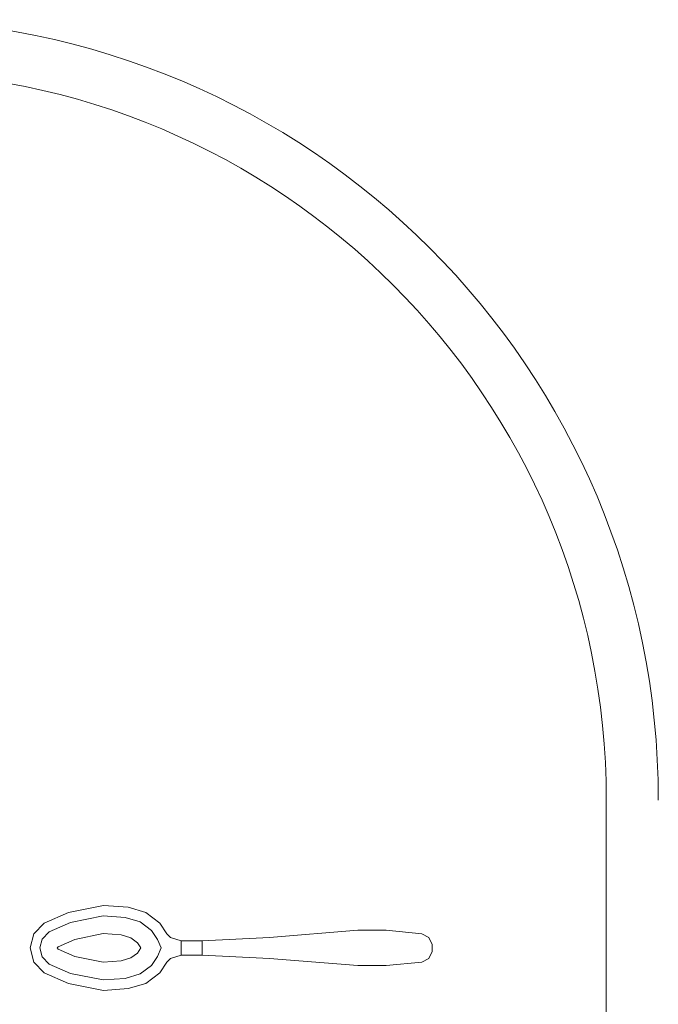
# Model space of a CAD drawing. Units: inches. Extents: x 375 to 1122, y 27 to 1069.
# Tile 147 of 155: x 737.5 to 747.02, y 901.85 to 916.52. Entities that reach past the tile are written whole.
import ezdxf

# ---------------------------------------------------------------- set-up
doc = ezdxf.new("R2010")
doc.units = ezdxf.units.IN
doc.layers.add('A-ANNO-DIMS', color=2, linetype='Continuous', lineweight=18)
doc.layers.add('Furniture', color=30, linetype='Continuous', lineweight=18)
doc.styles.get("Standard").update_dxf_attribs({"font": 'arial.ttf'})
doc.dimstyles.new('ISO-25', dxfattribs={"dimtxt": 12, "dimasz": 2.5, "dimexe": 1.5, "dimexo": 1.5, "dimtad": 1, "dimdec": 1, "dimlunit": 3, "dimtxsty": 'Standard', "dimblk": 'ARCHTICK', "dimcen": 2.5, "dimadec": 0, "dimazin": 0, "dimtfac": 1, "dimtdec": 1, "dimtmove": 0, "dimatfit": 3, "dimfxl": 1.5, "dimfxlon": 1, "dimarcsym": 0})

# ---------------------------------------------------------------- blocks, each defined once
blk = doc.blocks.new('A$C403C54AD')
blk.add_line((0.83575, 1.53256, -0.0006), (1.99923, 1.53256, -0.0006))
for radius in [0.29087, 0.27148]:
    blk.add_arc((0.83575, 1.26108, -0.0006), radius, 90, 180)
for points, invisible_edges in [([(0.88693, 1.46634, -0.04237), (0.89484, 1.46634, -0.04237), (0.89616, 1.4637, -0.04257), (0.88561, 1.4637, -0.04257)], 5), ([(0.88693, 1.46634, -0.04634), (0.89484, 1.46634, -0.04634), (0.89616, 1.4637, -0.04655), (0.88561, 1.4637, -0.04655)], 5), ([(0.8922, 1.46766, -0.04251), (0.88956, 1.46766, -0.04251), (0.88693, 1.46634, -0.04237), (0.89484, 1.46634, -0.04237)], 4), ([(0.8922, 1.46766, -0.04605), (0.88956, 1.46766, -0.04605), (0.88693, 1.46634, -0.04634), (0.89484, 1.46634, -0.04634)], 4), ([(0.89616, 1.4637, -0.04257), (0.88561, 1.4637, -0.04257), (0.88429, 1.45051, -0.0426), (0.89748, 1.45051, -0.0426)], 5), ([(0.89616, 1.4637, -0.04655), (0.88561, 1.4637, -0.04655), (0.88429, 1.45051, -0.04658), (0.89748, 1.45051, -0.04658)], 5), ([(0.88429, 1.45051, -0.0426), (0.89748, 1.45051, -0.0426), (0.89748, 1.43995, -0.04232), (0.88429, 1.43995, -0.04232)], 5), ([(0.88429, 1.45051, -0.04658), (0.89748, 1.45051, -0.04658), (0.89748, 1.43995, -0.0463), (0.88429, 1.43995, -0.0463)], 5), ([(0.89748, 1.43995, -0.0463), (0.88429, 1.43995, -0.0463), (0.88693, 1.40697, -0.04292), (0.89484, 1.40697, -0.04292)], 5), ([(0.88429, 1.43995, -0.0463), (0.88429, 1.43995, -0.04232), (0.88693, 1.40697, -0.04028), (0.88693, 1.40697, -0.04292)], 4), ([(0.89748, 1.43995, -0.04232), (0.88429, 1.43995, -0.04232), (0.88693, 1.40697, -0.04028), (0.89484, 1.40697, -0.04028)], 5), ([(0.89484, 1.40697, -0.04292), (0.89484, 1.40697, -0.04028), (0.89748, 1.43995, -0.04232), (0.89748, 1.43995, -0.0463)], 1), ([(0.88693, 1.40697, -0.04028), (0.89484, 1.40697, -0.04028), (0.89352, 1.3819, -0.03779), (0.88825, 1.3819, -0.03779)], 1), ([(0.88693, 1.40697, -0.04028), (0.88693, 1.40697, -0.04292), (0.88825, 1.3819, -0.04001), (0.88825, 1.3819, -0.03779)], 5), ([(0.88693, 1.40697, -0.04292), (0.89484, 1.40697, -0.04292), (0.89352, 1.3819, -0.04001), (0.88825, 1.3819, -0.04001)], 1), ([(0.89352, 1.3819, -0.03779), (0.89352, 1.3819, -0.04001), (0.89484, 1.40697, -0.04292), (0.89484, 1.40697, -0.04028)], 5), ([(0.88825, 1.3819, -0.04001), (0.88825, 1.3819, -0.03779), (0.88825, 1.37399, -0.03842), (0.88825, 1.37399, -0.04064)], 5), ([(0.89352, 1.37399, -0.04064), (0.89352, 1.37399, -0.03842), (0.89352, 1.3819, -0.03779), (0.89352, 1.3819, -0.04001)], 5), ([(0.88825, 1.37399, -0.03842), (0.89352, 1.37399, -0.03842), (0.89484, 1.37003, -0.04027), (0.88693, 1.37003, -0.04027)], 4), ([(0.88825, 1.37399, -0.03842), (0.88825, 1.37399, -0.04064), (0.88693, 1.37003, -0.04236), (0.88693, 1.37003, -0.04027)], 5), ([(0.88825, 1.37399, -0.04064), (0.89352, 1.37399, -0.04064), (0.89484, 1.37003, -0.04236), (0.88693, 1.37003, -0.04236)], 4), ([(0.89352, 1.37399, -0.04064), (0.89352, 1.37399, -0.03842), (0.89484, 1.37003, -0.04027), (0.89484, 1.37003, -0.04236)], 5), ([(0.89484, 1.37003, -0.04027), (0.88693, 1.37003, -0.04027), (0.88561, 1.3687, -0.041), (0.89616, 1.3687, -0.041)], 5), ([(0.89484, 1.37003, -0.04236), (0.88693, 1.37003, -0.04236), (0.88561, 1.3687, -0.04315), (0.89616, 1.3687, -0.04315)], 5), ([(0.88693, 1.37003, -0.04236), (0.88693, 1.37003, -0.04027), (0.88561, 1.3687, -0.041), (0.88561, 1.3687, -0.04315)], 1), ([(0.89484, 1.37003, -0.04027), (0.89484, 1.37003, -0.04236), (0.89616, 1.3687, -0.04315), (0.89616, 1.3687, -0.041)], 1), ([(0.88165, 1.36608, -0.04195), (0.88434, 1.36289, -0.04423), (0.88119, 1.35867, -0.04406), (0.87769, 1.36082, -0.04147)], 5), ([(0.88165, 1.36608, -0.04063), (0.88434, 1.36289, -0.04291), (0.88119, 1.35867, -0.04274), (0.87769, 1.36082, -0.04015)], 5), ([(0.88774, 1.36518, -0.04424), (0.88561, 1.3687, -0.04315), (0.88165, 1.36608, -0.04195), (0.88434, 1.36289, -0.04423)], 5), ([(0.88774, 1.36518, -0.04292), (0.88561, 1.3687, -0.041), (0.88165, 1.36608, -0.04063), (0.88434, 1.36289, -0.04291)], 5), ([(0.88561, 1.3687, -0.04315), (0.89088, 1.3687, -0.04315), (0.89088, 1.36654, -0.04406), (0.88774, 1.36518, -0.04424)], 11), ([(0.88561, 1.3687, -0.041), (0.89088, 1.3687, -0.041), (0.89088, 1.36654, -0.04274), (0.88774, 1.36518, -0.04292)], 11), ([(0.88774, 1.36518, -0.04424), (0.89088, 1.35902, -0.04627), (0.89088, 1.35902, -0.04627), (0.89088, 1.36654, -0.04406)], 5), ([(0.88774, 1.36518, -0.04292), (0.89088, 1.35902, -0.04495), (0.89088, 1.35902, -0.04495), (0.89088, 1.36654, -0.04274)], 5), ([(0.89616, 1.3687, -0.04315), (0.89088, 1.3687, -0.04315), (0.89088, 1.36654, -0.04406), (0.89402, 1.36518, -0.04424)], 11), ([(0.89616, 1.3687, -0.041), (0.89088, 1.3687, -0.041), (0.89088, 1.36654, -0.04274), (0.89402, 1.36518, -0.04292)], 11), ([(0.89402, 1.36518, -0.04424), (0.89088, 1.35902, -0.04627), (0.89088, 1.35902, -0.04627), (0.89088, 1.36654, -0.04406)], 5), ([(0.89402, 1.36518, -0.04292), (0.89088, 1.35902, -0.04495), (0.89088, 1.35902, -0.04495), (0.89088, 1.36654, -0.04274)], 5), ([(0.89402, 1.36518, -0.04292), (0.89616, 1.3687, -0.041), (0.90012, 1.36608, -0.04063), (0.89743, 1.36289, -0.04291)], 5), ([(0.90012, 1.36608, -0.04195), (0.89743, 1.36289, -0.04423), (0.90058, 1.35867, -0.04406), (0.90408, 1.36082, -0.04147)], 5), ([(0.90012, 1.36608, -0.04063), (0.89743, 1.36289, -0.04291), (0.90058, 1.35867, -0.04274), (0.90408, 1.36082, -0.04015)], 5), ([(0.88119, 1.35867, -0.04406), (0.88715, 1.3553, -0.04638), (0.88892, 1.35767, -0.04647), (0.88434, 1.36289, -0.04423)], 5), ([(0.88119, 1.35867, -0.04274), (0.88715, 1.3553, -0.04506), (0.88892, 1.35767, -0.04515), (0.88434, 1.36289, -0.04291)], 5), ([(0.88892, 1.35767, -0.04647), (0.88434, 1.36289, -0.04423), (0.88774, 1.36518, -0.04424), (0.89088, 1.35902, -0.04627)], 5), ([(0.88892, 1.35767, -0.04515), (0.88434, 1.36289, -0.04291), (0.88774, 1.36518, -0.04292), (0.89088, 1.35902, -0.04495)], 5), ([(0.89284, 1.35767, -0.04647), (0.89743, 1.36289, -0.04423), (0.89402, 1.36518, -0.04424), (0.89088, 1.35902, -0.04627)], 5), ([(0.89284, 1.35767, -0.04515), (0.89743, 1.36289, -0.04291), (0.89402, 1.36518, -0.04292), (0.89088, 1.35902, -0.04495)], 5), ([(0.90058, 1.35867, -0.04406), (0.89462, 1.3553, -0.04638), (0.89284, 1.35767, -0.04647), (0.89743, 1.36289, -0.04423)], 5), ([(0.90058, 1.35867, -0.04274), (0.89462, 1.3553, -0.04506), (0.89284, 1.35767, -0.04515), (0.89743, 1.36289, -0.04291)], 5), ([(0.88119, 1.35867, -0.04274), (0.87769, 1.36082, -0.04015), (0.87571, 1.35422, -0.03974), (0.87953, 1.35316, -0.04222)], 5), ([(0.88119, 1.35867, -0.04406), (0.87769, 1.36082, -0.04147), (0.87571, 1.35422, -0.04106), (0.87953, 1.35316, -0.04354)], 5), ([(0.88604, 1.35158, -0.04614), (0.87953, 1.35316, -0.04354), (0.88119, 1.35867, -0.04406), (0.88715, 1.3553, -0.04638)], 5), ([(0.88604, 1.35158, -0.04482), (0.87953, 1.35316, -0.04222), (0.88119, 1.35867, -0.04274), (0.88715, 1.3553, -0.04506)], 5), ([(0.88892, 1.35767, -0.04647), (0.89284, 1.35767, -0.04647), (0.89088, 1.35902, -0.04627)], 1), ([(0.88892, 1.35767, -0.04515), (0.89284, 1.35767, -0.04515), (0.89088, 1.35902, -0.04495)], 1), ([(0.89573, 1.35158, -0.04482), (0.90224, 1.35316, -0.04222), (0.90058, 1.35867, -0.04274), (0.89462, 1.3553, -0.04506)], 5), ([(0.90058, 1.35867, -0.04274), (0.90408, 1.36082, -0.04015), (0.90606, 1.35422, -0.03974), (0.90224, 1.35316, -0.04222)], 5), ([(0.90058, 1.35867, -0.04406), (0.90408, 1.36082, -0.04147), (0.90606, 1.35422, -0.04106), (0.90224, 1.35316, -0.04354)], 5), ([(0.88604, 1.35158, -0.04614), (0.89573, 1.35158, -0.04614), (0.89462, 1.3553, -0.04638), (0.88715, 1.3553, -0.04638)], 5), ([(0.88604, 1.35158, -0.04482), (0.89573, 1.35158, -0.04482), (0.89462, 1.3553, -0.04506), (0.88715, 1.3553, -0.04506)], 5), ([(0.89462, 1.3553, -0.04638), (0.88715, 1.3553, -0.04638), (0.88892, 1.35767, -0.04647), (0.89284, 1.35767, -0.04647)], 5), ([(0.89462, 1.3553, -0.04506), (0.88715, 1.3553, -0.04506), (0.88892, 1.35767, -0.04515), (0.89284, 1.35767, -0.04515)], 5), ([(0.87571, 1.35422, -0.03974), (0.87953, 1.35316, -0.04222), (0.87893, 1.34491, -0.04133), (0.87505, 1.34501, -0.03888)], 5), ([(0.87571, 1.35422, -0.04106), (0.87953, 1.35316, -0.04354), (0.87893, 1.34491, -0.04265), (0.87505, 1.34501, -0.0402)], 5), ([(0.87893, 1.34491, -0.04265), (0.88556, 1.34497, -0.0452), (0.88604, 1.35158, -0.04614), (0.87953, 1.35316, -0.04354)], 5), ([(0.87893, 1.34491, -0.04133), (0.88556, 1.34497, -0.04388), (0.88604, 1.35158, -0.04482), (0.87953, 1.35316, -0.04222)], 5), ([(0.89621, 1.34497, -0.0452), (0.88556, 1.34497, -0.0452), (0.88604, 1.35158, -0.04614), (0.89573, 1.35158, -0.04614)], 5), ([(0.89621, 1.34497, -0.04388), (0.88556, 1.34497, -0.04388), (0.88604, 1.35158, -0.04482), (0.89573, 1.35158, -0.04482)], 5), ([(0.90283, 1.34491, -0.04265), (0.89621, 1.34497, -0.0452), (0.89573, 1.35158, -0.04614), (0.90224, 1.35316, -0.04354)], 5), ([(0.90283, 1.34491, -0.04133), (0.89621, 1.34497, -0.04388), (0.89573, 1.35158, -0.04482), (0.90224, 1.35316, -0.04222)], 5), ([(0.90606, 1.35422, -0.03974), (0.90224, 1.35316, -0.04222), (0.90283, 1.34491, -0.04133), (0.90672, 1.34501, -0.03888)], 5), ([(0.90606, 1.35422, -0.04106), (0.90224, 1.35316, -0.04354), (0.90283, 1.34491, -0.04265), (0.90672, 1.34501, -0.0402)], 5), ([(0.87893, 1.34491, -0.04265), (0.87505, 1.34501, -0.0402), (0.87769, 1.33198, -0.03816), (0.88139, 1.33278, -0.04067)], 5), ([(0.87893, 1.34491, -0.04133), (0.87505, 1.34501, -0.03888), (0.87769, 1.33198, -0.03684), (0.88139, 1.33278, -0.03935)], 5), ([(0.88771, 1.33436, -0.04216), (0.88139, 1.33278, -0.03935), (0.87893, 1.34491, -0.04133), (0.88556, 1.34497, -0.04388)], 5), ([(0.88771, 1.33436, -0.04348), (0.88139, 1.33278, -0.04067), (0.87893, 1.34491, -0.04265), (0.88556, 1.34497, -0.0452)], 5), ([(0.88771, 1.33436, -0.04216), (0.89406, 1.33436, -0.04216), (0.89621, 1.34497, -0.04388), (0.88556, 1.34497, -0.04388)], 5), ([(0.88771, 1.33436, -0.04348), (0.89406, 1.33436, -0.04348), (0.89621, 1.34497, -0.0452), (0.88556, 1.34497, -0.0452)], 5), ([(0.89406, 1.33436, -0.04216), (0.90038, 1.33278, -0.03935), (0.90283, 1.34491, -0.04133), (0.89621, 1.34497, -0.04388)], 5), ([(0.89406, 1.33436, -0.04348), (0.90038, 1.33278, -0.04067), (0.90283, 1.34491, -0.04265), (0.89621, 1.34497, -0.0452)], 5), ([(0.90283, 1.34491, -0.04265), (0.90672, 1.34501, -0.0402), (0.90408, 1.33198, -0.03816), (0.90038, 1.33278, -0.04067)], 5), ([(0.90283, 1.34491, -0.04133), (0.90672, 1.34501, -0.03888), (0.90408, 1.33198, -0.03684), (0.90038, 1.33278, -0.03935)], 5), ([(0.87769, 1.33198, -0.03816), (0.88139, 1.33278, -0.04067), (0.8849, 1.32476, -0.03896), (0.88165, 1.32291, -0.03632)], 5), ([(0.87769, 1.33198, -0.03684), (0.88139, 1.33278, -0.03935), (0.8849, 1.32476, -0.03764), (0.88165, 1.32291, -0.035)], 5), ([(0.8849, 1.32476, -0.03896), (0.89045, 1.32814, -0.04186), (0.88771, 1.33436, -0.04348), (0.88139, 1.33278, -0.04067)], 5), ([(0.8849, 1.32476, -0.03764), (0.89045, 1.32814, -0.04054), (0.88771, 1.33436, -0.04216), (0.88139, 1.33278, -0.03935)], 5), ([(0.89132, 1.32814, -0.04186), (0.89045, 1.32814, -0.04186), (0.88771, 1.33436, -0.04348), (0.89406, 1.33436, -0.04348)], 5), ([(0.89132, 1.32814, -0.04054), (0.89045, 1.32814, -0.04054), (0.88771, 1.33436, -0.04216), (0.89406, 1.33436, -0.04216)], 5), ([(0.89687, 1.32476, -0.03896), (0.89132, 1.32814, -0.04186), (0.89406, 1.33436, -0.04348), (0.90038, 1.33278, -0.04067)], 5), ([(0.89687, 1.32476, -0.03764), (0.89132, 1.32814, -0.04054), (0.89406, 1.33436, -0.04216), (0.90038, 1.33278, -0.03935)], 5), ([(0.90408, 1.33198, -0.03816), (0.90038, 1.33278, -0.04067), (0.89687, 1.32476, -0.03896), (0.90012, 1.32291, -0.03632)], 5), ([(0.90408, 1.33198, -0.03684), (0.90038, 1.33278, -0.03935), (0.89687, 1.32476, -0.03764), (0.90012, 1.32291, -0.035)], 5), ([(0.89045, 1.32814, -0.04054), (0.88758, 1.32213, -0.03709), (0.8849, 1.32476, -0.03764), (0.89045, 1.32814, -0.04054)], 5), ([(0.89045, 1.32814, -0.04186), (0.88758, 1.32213, -0.03841), (0.8849, 1.32476, -0.03896), (0.89045, 1.32814, -0.04186)], 5), ([(0.89088, 1.32132, -0.0369), (0.89088, 1.32772, -0.0404), (0.89045, 1.32814, -0.04054), (0.88758, 1.32213, -0.03709)], 5), ([(0.89088, 1.32132, -0.03822), (0.89088, 1.32772, -0.04172), (0.89045, 1.32814, -0.04186), (0.88758, 1.32213, -0.03841)], 5), ([(0.89088, 1.32772, -0.0404), (0.89045, 1.32814, -0.04054), (0.89132, 1.32814, -0.04054), (0.89088, 1.32772, -0.0404)], 2), ([(0.89088, 1.32772, -0.04172), (0.89045, 1.32814, -0.04186), (0.89132, 1.32814, -0.04186), (0.89088, 1.32772, -0.04172)], 2), ([(0.89088, 1.32132, -0.0369), (0.89088, 1.32772, -0.0404), (0.89132, 1.32814, -0.04054), (0.89419, 1.32213, -0.03709)], 5), ([(0.89088, 1.32132, -0.03822), (0.89088, 1.32772, -0.04172), (0.89132, 1.32814, -0.04186), (0.89419, 1.32213, -0.03841)], 5), ([(0.89132, 1.32814, -0.04054), (0.89419, 1.32213, -0.03709), (0.89687, 1.32476, -0.03764), (0.89132, 1.32814, -0.04054)], 5), ([(0.89132, 1.32814, -0.04186), (0.89419, 1.32213, -0.03841), (0.89687, 1.32476, -0.03896), (0.89132, 1.32814, -0.04186)], 5), ([(0.8849, 1.32476, -0.03896), (0.88165, 1.32291, -0.03632), (0.88561, 1.31907, -0.03523), (0.88758, 1.32213, -0.03841)], 5), ([(0.8849, 1.32476, -0.03764), (0.88165, 1.32291, -0.035), (0.88561, 1.31907, -0.03391), (0.88758, 1.32213, -0.03709)], 5), ([(0.88561, 1.31907, -0.03523), (0.88758, 1.32213, -0.03841), (0.89088, 1.32132, -0.03822), (0.89088, 1.31776, -0.03505)], 5), ([(0.88561, 1.31907, -0.03391), (0.88758, 1.32213, -0.03709), (0.89088, 1.32132, -0.0369), (0.89088, 1.31776, -0.03373)], 5), ([(0.89616, 1.31907, -0.03523), (0.89419, 1.32213, -0.03841), (0.89088, 1.32132, -0.03822), (0.89088, 1.31776, -0.03505)], 5), ([(0.89616, 1.31907, -0.03391), (0.89419, 1.32213, -0.03709), (0.89088, 1.32132, -0.0369), (0.89088, 1.31776, -0.03373)], 5), ([(0.89687, 1.32476, -0.03896), (0.90012, 1.32291, -0.03632), (0.89616, 1.31907, -0.03523), (0.89419, 1.32213, -0.03841)], 5), ([(0.89687, 1.32476, -0.03764), (0.90012, 1.32291, -0.035), (0.89616, 1.31907, -0.03391), (0.89419, 1.32213, -0.03709)], 5)]:
    blk.add_3dface(points, dxfattribs=dict(invisible_edges=invisible_edges))
for points in [[(0.88693, 1.46634, -0.04237), (0.88693, 1.46634, -0.04634), (0.88561, 1.4637, -0.04655), (0.88561, 1.4637, -0.04257)], [(0.88956, 1.46766, -0.04605), (0.88956, 1.46766, -0.04251), (0.88693, 1.46634, -0.04237), (0.88693, 1.46634, -0.04634)], [(0.8922, 1.46766, -0.04251), (0.8922, 1.46766, -0.04605), (0.88956, 1.46766, -0.04605), (0.88956, 1.46766, -0.04251)], [(0.89484, 1.46634, -0.04634), (0.89484, 1.46634, -0.04237), (0.8922, 1.46766, -0.04251), (0.8922, 1.46766, -0.04605)], [(0.89616, 1.4637, -0.04257), (0.89616, 1.4637, -0.04655), (0.89484, 1.46634, -0.04634), (0.89484, 1.46634, -0.04237)], [(0.88561, 1.4637, -0.04655), (0.88561, 1.4637, -0.04257), (0.88429, 1.45051, -0.0426), (0.88429, 1.45051, -0.04658)], [(0.89748, 1.45051, -0.04658), (0.89748, 1.45051, -0.0426), (0.89616, 1.4637, -0.04257), (0.89616, 1.4637, -0.04655)], [(0.88429, 1.45051, -0.0426), (0.88429, 1.45051, -0.04658), (0.88429, 1.43995, -0.0463), (0.88429, 1.43995, -0.04232)], [(0.89748, 1.43995, -0.04232), (0.89748, 1.43995, -0.0463), (0.89748, 1.45051, -0.04658), (0.89748, 1.45051, -0.0426)], [(0.89352, 1.3819, -0.04001), (0.88825, 1.3819, -0.04001), (0.88825, 1.37399, -0.04064), (0.89352, 1.37399, -0.04064)], [(0.89352, 1.3819, -0.03779), (0.88825, 1.3819, -0.03779), (0.88825, 1.37399, -0.03842), (0.89352, 1.37399, -0.03842)], [(0.88165, 1.36608, -0.04063), (0.88165, 1.36608, -0.04195), (0.87769, 1.36082, -0.04147), (0.87769, 1.36082, -0.04015)], [(0.88561, 1.3687, -0.04315), (0.88561, 1.3687, -0.041), (0.88165, 1.36608, -0.04063), (0.88165, 1.36608, -0.04195)], [(0.90012, 1.36608, -0.04195), (0.90012, 1.36608, -0.04063), (0.89616, 1.3687, -0.041), (0.89616, 1.3687, -0.04315)], [(0.90408, 1.36082, -0.04015), (0.90408, 1.36082, -0.04147), (0.90012, 1.36608, -0.04195), (0.90012, 1.36608, -0.04063)], [(0.87769, 1.36082, -0.04147), (0.87769, 1.36082, -0.04015), (0.87571, 1.35422, -0.03974), (0.87571, 1.35422, -0.04106)], [(0.90606, 1.35422, -0.04106), (0.90606, 1.35422, -0.03974), (0.90408, 1.36082, -0.04015), (0.90408, 1.36082, -0.04147)], [(0.87571, 1.35422, -0.03974), (0.87571, 1.35422, -0.04106), (0.87505, 1.34501, -0.0402), (0.87505, 1.34501, -0.03888)], [(0.90672, 1.34501, -0.0402), (0.90672, 1.34501, -0.03888), (0.90606, 1.35422, -0.03974), (0.90606, 1.35422, -0.04106)], [(0.87505, 1.34501, -0.0402), (0.87505, 1.34501, -0.03888), (0.87769, 1.33198, -0.03684), (0.87769, 1.33198, -0.03816)], [(0.90408, 1.33198, -0.03684), (0.90408, 1.33198, -0.03816), (0.90672, 1.34501, -0.0402), (0.90672, 1.34501, -0.03888)], [(0.87769, 1.33198, -0.03684), (0.87769, 1.33198, -0.03816), (0.88165, 1.32291, -0.03632), (0.88165, 1.32291, -0.035)], [(0.90012, 1.32291, -0.03632), (0.90012, 1.32291, -0.035), (0.90408, 1.33198, -0.03684), (0.90408, 1.33198, -0.03816)], [(0.88165, 1.32291, -0.03632), (0.88165, 1.32291, -0.035), (0.88561, 1.31907, -0.03391), (0.88561, 1.31907, -0.03523)], [(0.89616, 1.31907, -0.03391), (0.89616, 1.31907, -0.03523), (0.90012, 1.32291, -0.03632), (0.90012, 1.32291, -0.035)], [(0.88561, 1.31907, -0.03391), (0.88561, 1.31907, -0.03523), (0.89088, 1.31776, -0.03505), (0.89088, 1.31776, -0.03373)], [(0.89088, 1.31776, -0.03505), (0.89088, 1.31776, -0.03373), (0.89616, 1.31907, -0.03391), (0.89616, 1.31907, -0.03523)]]:
    blk.add_3dface(points)
blk = doc.blocks.new('_ArchTick')
at = {"color": 0, "linetype": 'ByBlock', "const_width": 0.15}
blk.add_lwpolyline([(-0.5, -0.5), (0.5, 0.5)], dxfattribs=at)
blk = doc.blocks.new('*D73')
at = {"layer": 'A-ANNO-DIMS', "color": 0, "lineweight": -2, "transparency": 16777216}
for p, q in [((686.757, 932.428), (686.757, 929.428)), ((770.757, 932.428), (770.757, 929.428)), ((686.757, 930.928), (770.757, 930.928)), ((770.757, 930.928), (987.61, 930.928))]:
    blk.add_line(p, q, dxfattribs=at)
at = {"layer": 'Defpoints', "color": 0, "transparency": 16777216}
for p in [(686.757, 943.528), (770.757, 943.528), (770.757, 930.928)]:
    blk.add_point(p, dxfattribs=at)
at = {"layer": 'A-ANNO-DIMS', "color": 0, "lineweight": -2, "transparency": 16777216, "xscale": 2.5, "yscale": 2.5, "zscale": 2.5, "rotation": 180}
blk.add_blockref('_ArchTick', (686.757, 930.928), dxfattribs=at)
at = {"layer": 'A-ANNO-DIMS', "color": 0, "lineweight": -2, "transparency": 16777216, "xscale": 2.5, "yscale": 2.5, "zscale": 2.5}
blk.add_blockref('_ArchTick', (770.757, 930.928), dxfattribs=at)
at = {"layer": 'A-ANNO-DIMS', "color": 0, "transparency": 16777216, "insert": (880.433, 937.757), "char_height": 12, "attachment_point": 5}
blk.add_mtext('2-PANEL SLIDER 7\'-0" TYP.', dxfattribs=at)
blk = doc.blocks.new('*D88')
at = {"layer": 'A-ANNO-DIMS', "color": 0, "lineweight": -2, "transparency": 16777216}
for p, q in [((731.007, 1052.528), (731.007, 1055.528)), ((854.007, 1052.528), (854.007, 1055.528)), ((731.007, 1054.028), (854.007, 1054.028))]:
    blk.add_line(p, q, dxfattribs=at)
at = {"layer": 'Defpoints', "color": 0, "transparency": 16777216}
for p in [(854.007, 1054.028), (731.007, 502.528), (854.007, 502.528)]:
    blk.add_point(p, dxfattribs=at)
at = {"layer": 'A-ANNO-DIMS', "color": 0, "lineweight": -2, "transparency": 16777216, "xscale": 2.5, "yscale": 2.5, "zscale": 2.5, "rotation": 180}
blk.add_blockref('_ArchTick', (731.007, 1054.028), dxfattribs=at)
at = {"layer": 'A-ANNO-DIMS', "color": 0, "lineweight": -2, "transparency": 16777216, "xscale": 2.5, "yscale": 2.5, "zscale": 2.5}
blk.add_blockref('_ArchTick', (854.007, 1054.028), dxfattribs=at)
at = {"layer": 'A-ANNO-DIMS', "color": 0, "transparency": 16777216, "insert": (792.507, 1060.784), "char_height": 12, "attachment_point": 5}
blk.add_mtext('10\'-3"', dxfattribs=at)
blk = doc.blocks.new('*D91')
at = {"layer": 'A-ANNO-DIMS', "color": 0, "lineweight": -2, "transparency": 16777216}
for p, q in [((728.007, 1052.528), (728.007, 1055.528)), ((788.007, 1052.528), (788.007, 1055.528)), ((728.007, 1054.028), (788.007, 1054.028))]:
    blk.add_line(p, q, dxfattribs=at)
at = {"layer": 'Defpoints', "color": 0, "transparency": 16777216}
for p in [(788.007, 1054.028), (728.007, 774.028), (788.007, 774.028)]:
    blk.add_point(p, dxfattribs=at)
at = {"layer": 'A-ANNO-DIMS', "color": 0, "lineweight": -2, "transparency": 16777216, "xscale": 2.5, "yscale": 2.5, "zscale": 2.5, "rotation": 180}
blk.add_blockref('_ArchTick', (728.007, 1054.028), dxfattribs=at)
at = {"layer": 'A-ANNO-DIMS', "color": 0, "lineweight": -2, "transparency": 16777216, "xscale": 2.5, "yscale": 2.5, "zscale": 2.5}
blk.add_blockref('_ArchTick', (788.007, 1054.028), dxfattribs=at)
at = {"layer": 'A-ANNO-DIMS', "color": 0, "transparency": 16777216, "insert": (758.007, 1060.78), "char_height": 12, "attachment_point": 5}
blk.add_mtext('5\'-0"', dxfattribs=at)

msp = doc.modelspace()

# ---------------------------------------------------------------- block references
at = {"layer": 'Furniture', "xscale": 39.9918517141215, "yscale": 39.9918517141215, "zscale": 39.9918517141215, "rotation": 270}
msp.add_blockref('A$C403C54AD', (684.955, 938.316, 0.024), dxfattribs=at)

# ---------------------------------------------------------------- dimensions: what is measured, and where the dimension line sits
at = {"layer": 'A-ANNO-DIMS'}
for base, p1, p2, picture, middle in [((788.007, 1054.028), (728.007, 774.028), (788.007, 774.028), '*D91', (758.007, 1060.78)), ((854.007, 1054.028), (731.007, 502.528), (854.007, 502.528), '*D88', (792.507, 1060.784))]:
    dim = msp.add_linear_dim(base=base, p1=p1, p2=p2, dimstyle='ISO-25', override={"dimdec": 1, "dimlfac": 1, "dimrnd": 0, "dimzin": 1, "dimdsep": 46, "dimlunit": 4, "dimfrac": 2}, dxfattribs=at)
    dim.commit()
    dim.dimension.update_dxf_attribs({"geometry": picture, "text_midpoint": middle})
dim = msp.add_linear_dim(base=(770.757, 930.928), p1=(686.757, 943.528), p2=(770.757, 943.528), text='2-PANEL SLIDER <> TYP.', dimstyle='ISO-25', override={"dimdec": 1, "dimlfac": 1, "dimrnd": 0, "dimzin": 1, "dimdsep": 46, "dimlunit": 4, "dimfrac": 2}, dxfattribs=at)
dim.commit()
dim.dimension.update_dxf_attribs({"geometry": '*D73', "text_midpoint": (880.433, 937.757)})

doc.saveas('drawing.dxf')
